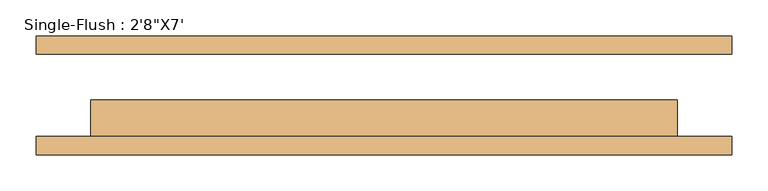
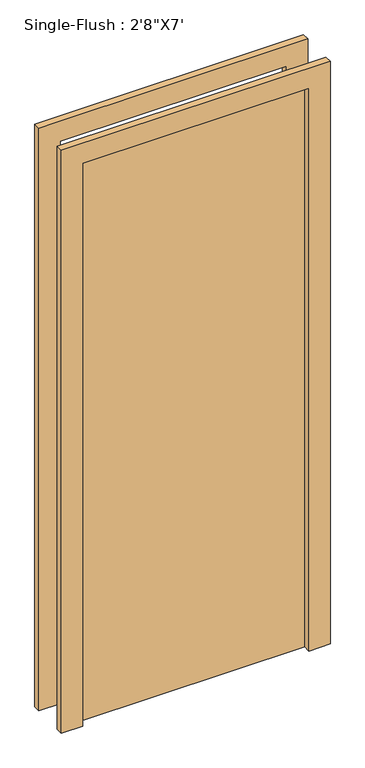
"""IFC4 building model written with IfcOpenShell, lengths in millimetres: door geometry."""

from ifc_helpers import new_model, si_unit, frame, origin, origin_with_axes, place, context, project, spatial, polyline, outline, extrude, source, transform, mapped, element, save


def door_38851409(model_context):
    return source(origin(), model_context, "Body", "SweptSolid", [
        extrude(outline(polyline([(2209.8, -482.6), (0.0, -482.6), (0.0, -406.4), (2133.6, -406.4), (2133.6, 406.4), (0.0, 406.4), (0.0, 482.6), (2209.8, 482.6), (2209.8, -482.6)])), frame((0.0, -82.55, 0.0), z_axis=(0.0, 1.0, 0.0), x_axis=(0.0, 0.0, 1.0)), (0.0, 0.0, 1.0), 25.4),
        extrude(outline(polyline([(2209.8, 482.6), (2209.8, -482.6), (0.0, -482.6), (0.0, -406.4), (2133.6, -406.4), (2133.6, 406.4), (0.0, 406.4), (0.0, 482.6), (2209.8, 482.6)])), frame((0.0, 57.15, 0.0), z_axis=(0.0, 1.0, 0.0), x_axis=(0.0, 0.0, 1.0)), (0.0, 0.0, 1.0), 25.4),
        extrude(outline(polyline([(406.4, -6.35), (406.4, -57.15), (-406.4, -57.15), (-406.4, -6.35), (406.4, -6.35)])), origin_with_axes(), (0.0, 0.0, 1.0), 2133.6),
    ])


if __name__ == "__main__":
    model = new_model("IFC4")
    model_context = context("Model", 3, world=origin())
    ifc_project = project(units=[si_unit("LENGTHUNIT", "METRE", prefix="MILLI")], contexts=[model_context])
    site = spatial("IfcSite", under=ifc_project)
    building = spatial("IfcBuilding", under=site)
    placement = place(None, origin())
    door_shape = door_38851409(model_context)
    element("IfcDoor", 1, ObjectType="Single-Flush : 2'8\"X7'", at=placement, inside=building, context=model_context, shape_type="MappedRepresentation", body=[
        mapped(door_shape, transform((0.0, 0.0, 0.0), x_axis=(1.0, 0.0, 0.0), y_axis=(0.0, 1.0, 0.0), z_axis=(0.0, 0.0, 1.0))),
    ])
    save(model, "model.ifc")

# Revit data of these elements
# Type "Single-Flush : 2'8\"X7'"
#   Type Mark = "9"
#   Construction Type Id = "MDOOR"
#   Assembly Code = "C1020"
#   Analytic Construction = "Metal"
#   Thickness = 0' - 2"
#   Heat Transfer Coefficient (U) = 0.651978 BTU/(h·ft²·°F)
#   Height = 7' - 0"
#   Trim Projection Ext = 0' - 1"
#   Trim Projection Int = 0' - 1"
#   Trim Width = 0' - 3"
#   Width = 2' - 8"
#   Define Thermal Properties by = 1
#   Door Material = Door - Panel
#   Frame Material = Door - Frame
#   Visual Light Transmittance = 0
#   Solar Heat Gain Coefficient = 0
#   Function = (empty or 0)
#   Wall Closure = (empty or 0)
# Element 1 (IfcDoor, "Single-Flush : 2'8\"X7'")
#   Materials on its faces: "Door - Frame", "Door - Panel"
# Materials
#   "Door - Panel": class "Wood", colour RGB 210 159 95, transparency 0, Cost = 0
#   "Door - Frame": colour RGB 118 70 51, transparency 0, Cost = 0
